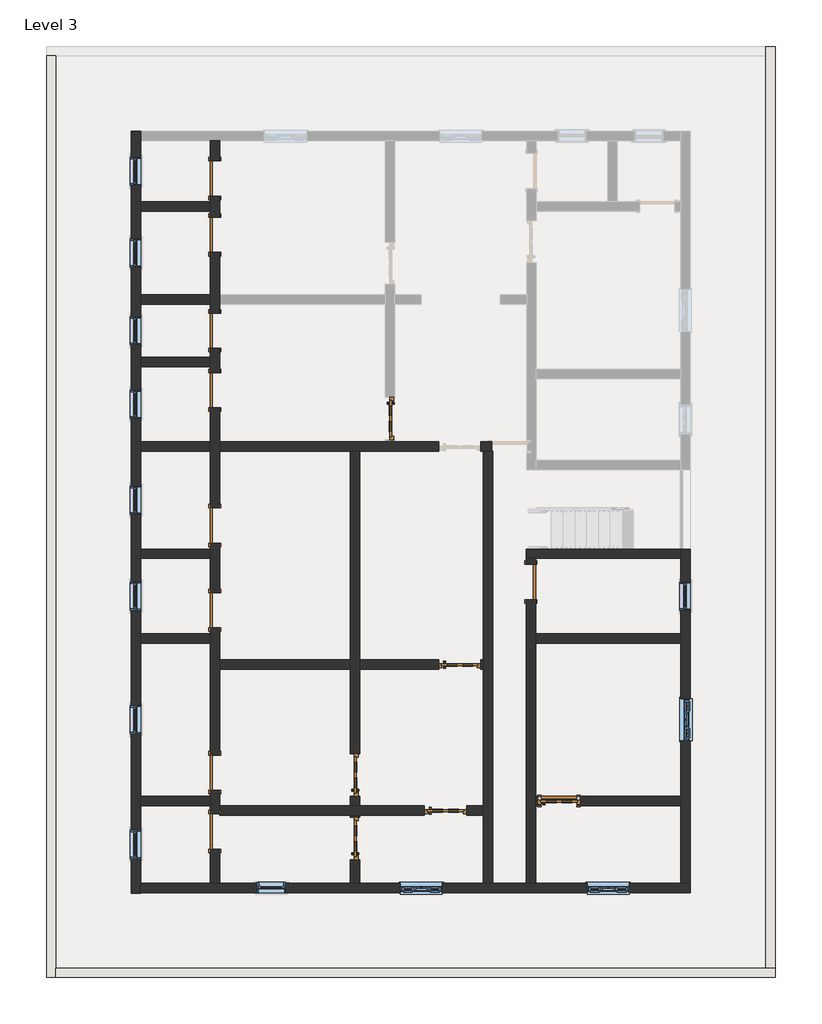
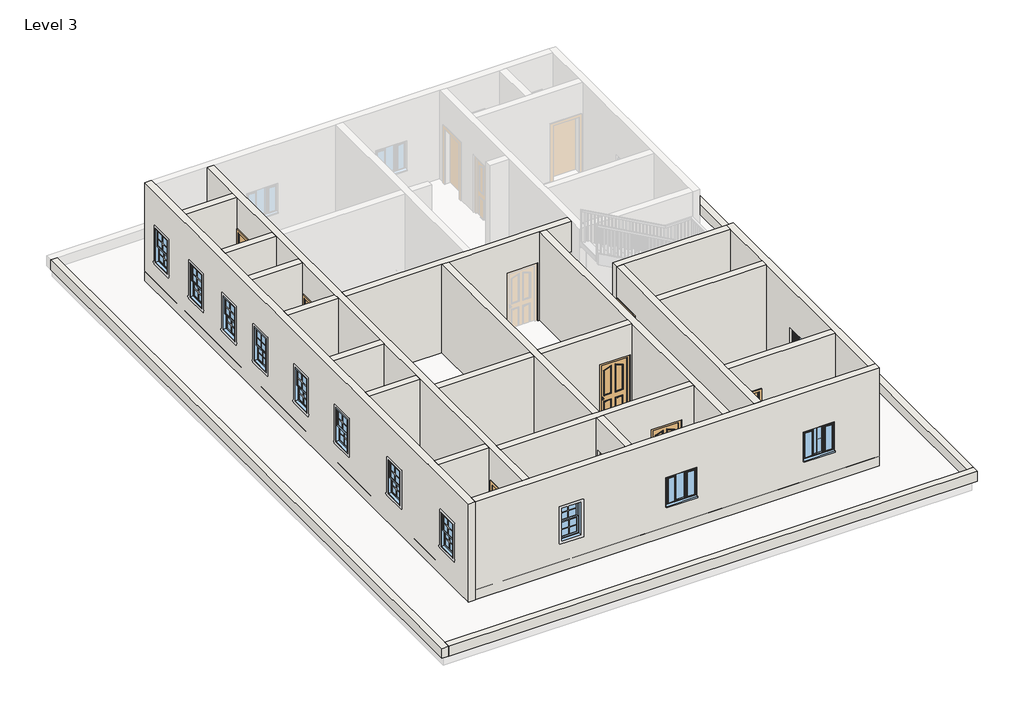
# One storey, part 1 of 3: 22 walls, 16 doors, 13 windows.
# Revit data of these elements (continued)
# Element 44 (IfcWindow, "Window-Double-Hung : 24\" x 42\"")
#   Mark = "47"
#   Window Inset = 0' - 0"
#   Interior Wall Closure = 0' - 1 1/2"
#   Frame Extension = 0' - 1 1/4"
#   Exterior Wall Closure = 0' - 0 1/2"
#   Interior Trim Visibility = yes
#   Indicator Visibility = yes
#   Exterior Trim Visibility = yes
#   Phase Created = New Construction
#   Materials on its faces: "Wood - Stained", "Glass", "Clad - White"
# Element 45 (IfcWindow, "Window-Double-Hung : 24\" x 42\"")
#   Mark = "48"
#   Window Inset = 0' - 0"
#   Interior Wall Closure = 0' - 1 1/2"
#   Frame Extension = 0' - 1 1/4"
#   Exterior Wall Closure = 0' - 0 1/2"
#   Interior Trim Visibility = yes
#   Indicator Visibility = yes
#   Exterior Trim Visibility = yes
#   Phase Created = New Construction
#   Materials on its faces: "Wood - Stained", "Glass", "Clad - White"
# Element 46 (IfcWindow, "Window-Double-Hung : 24\" x 42\"")
#   Mark = "49"
#   Window Inset = 0' - 0"
#   Interior Wall Closure = 0' - 1 1/2"
#   Frame Extension = 0' - 1 1/4"
#   Exterior Wall Closure = 0' - 0 1/2"
#   Interior Trim Visibility = yes
#   Indicator Visibility = yes
#   Exterior Trim Visibility = yes
#   Phase Created = New Construction
#   Materials on its faces: "Wood - Stained", "Glass", "Clad - White"
# Element 47 (IfcWindow, "Window-Double-Hung : 24\" x 42\"")
#   Mark = "50"
#   Window Inset = 0' - 0"
#   Interior Wall Closure = 0' - 1 1/2"
#   Frame Extension = 0' - 1 1/4"
#   Exterior Wall Closure = 0' - 0 1/2"
#   Interior Trim Visibility = yes
#   Indicator Visibility = yes
#   Exterior Trim Visibility = yes
#   Phase Created = New Construction
#   Materials on its faces: "Wood - Stained", "Glass", "Clad - White"
# Element 48 (IfcWindow, "Window-Double-Hung : 24\" x 42\"")
#   Mark = "51"
#   Window Inset = 0' - 0"
#   Interior Wall Closure = 0' - 1 1/2"
#   Frame Extension = 0' - 1 1/4"
#   Exterior Wall Closure = 0' - 0 1/2"
#   Interior Trim Visibility = yes
#   Indicator Visibility = yes
#   Exterior Trim Visibility = yes
#   Phase Created = New Construction
#   Materials on its faces: "Wood - Stained", "Glass", "Clad - White"
# Element 49 (IfcWindow, "Windows_Tpl_w-Glazing_Cross-Bars : 910x910mm")
#   Mark = "39"
#   Phase Created = New Construction
#   Materials on its faces: "Window Frame", "Glass"
# Element 50 (IfcWindow, "Windows_Tpl_w-Glazing_Cross-Bars : 910x910mm")
#   Mark = "56"
#   Phase Created = New Construction
#   Materials on its faces: "Window Frame", "Glass"
# Element 51 (IfcWindow, "Windows_Tpl_w-Glazing_Cross-Bars : 910x910mm")
#   Mark = "57"
#   Phase Created = New Construction
#   Materials on its faces: "Window Frame", "Glass"
# Materials
#   "Door - Glazing": colour RGB 0 0 255, transparency 0.75
#   "Door - Panel": class "Wood", colour RGB 210 159 95, transparency 0, Cost = 0
#   "Door - Frame/Mullion": class "Wood", colour RGB 212 179 113, transparency 0
#   "Door - Handle": colour RGB 246 240 166, transparency 0
#   "Door - Frame": colour RGB 118 70 51, transparency 0, Cost = 0
#   "Wood - Stained": class "Wood", colour RGB 224 178 126, transparency 0, Cost = 0
#   "Clad - White": class "Wood", colour RGB 242 242 238, transparency 0, Cost = 0
#   "Glass": class "Glass", colour RGB 0 128 192, transparency 0.75, Description = "Soda Lime Glass", Cost = 0
#   "Window Frame": colour RGB 249 249 249, transparency 0
#   "Default Wall": colour RGB 128 128 128, transparency 0, Cost = 0
#   "Tile, Porcelain, 4in": class "Generic", colour RGB 89 87 158, transparency 0, Description = "Porcelain tile, 4\", white", Cost = 0
